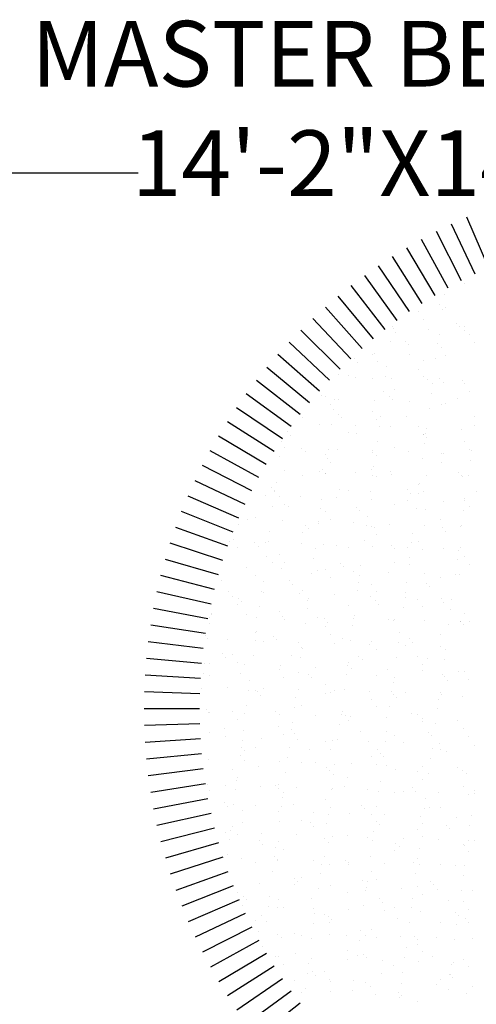
# Model space of a CAD drawing. Units: inches. Extents: x 1566 to 2546, y 1087 to 2705.
# Tile 16 of 27: x 2315 to 2364, y 1243 to 1348. Entities that reach past the tile are written whole.
import ezdxf

# ---------------------------------------------------------------- set-up
doc = ezdxf.new("R2010")
doc.units = ezdxf.units.IN
for name, color, linetype, lineweight in [('A-ANNO-DIMS', 2, 'Continuous', 18), ('A-AREA-IDEN', 7, 'Continuous', 18), ('A-FURN', 8, 'Continuous', 18)]:
    doc.layers.add(name, color=color, linetype=linetype, lineweight=lineweight)
doc.layers.add('A-HT', color=15, linetype='Continuous')
doc.styles.get("Standard").update_dxf_attribs({"font": 'arial.ttf'})
doc.dimstyles.new('ISO-25', dxfattribs={"dimtxt": 2.5, "dimasz": 2.5, "dimexe": 1.25, "dimexo": 0.625, "dimtad": 1, "dimtxsty": 'Standard', "dimcen": 2.5, "dimadec": 0, "dimazin": 0, "dimtfac": 1, "dimtmove": 0, "dimatfit": 3, "dimfxl": 1, "dimarcsym": 0})

# ---------------------------------------------------------------- blocks, each defined once
blk = doc.blocks.new('*X21')
at = {"color": 0}
for p, q in [((1.8017, 2.833), (1.8017, 2.833)), ((1.8104, 2.8275), (1.8104, 2.8275)), ((1.8783, 2.8364), (1.8783, 2.8364)), ((1.9044, 2.8399), (1.9044, 2.8399)), ((1.945, 2.8452), (1.945, 2.8452)), ((2.0018, 2.8313), (2.0018, 2.8313)), ((2.2048, 2.8269), (2.2048, 2.8269)), ((1.7428, 2.8186), (1.7428, 2.8186)), ((1.7438, 2.8187), (1.7438, 2.8187)), ((1.7537, 2.8227), (1.7537, 2.8227)), ((1.7698, 2.8221), (1.7698, 2.8221)), ((1.8778, 2.8235), (1.8778, 2.8235)), ((1.9094, 2.823), (1.9094, 2.823)), ((2.0087, 2.8252), (2.0087, 2.8252)), ((2.011, 2.8229), (2.011, 2.8229)), ((2.0652, 2.8233), (2.0652, 2.8233)), ((2.1366, 2.8246), (2.1366, 2.8246)), ((2.2209, 2.8236), (2.2209, 2.8236)), ((1.6514, 2.7891), (1.6514, 2.7891)), ((1.8133, 2.774), (1.8133, 2.774)), ((1.8515, 2.7874), (1.8515, 2.7874)), ((1.8607, 2.779), (1.8607, 2.779)), ((1.9412, 2.7734), (1.9412, 2.7734)), ((2.0545, 2.783), (2.0545, 2.783)), ((2.0763, 2.7783), (2.0763, 2.7783)), ((2.2072, 2.78), (2.2072, 2.78)), ((2.2546, 2.7813), (2.2546, 2.7813)), ((2.2638, 2.7728), (2.2638, 2.7728)), ((2.3351, 2.7793), (2.3351, 2.7793)), ((2.3949, 2.775), (2.3949, 2.775)), ((1.5414, 2.759), (1.5414, 2.759)), ((1.5474, 2.7675), (1.5474, 2.7675)), ((1.6825, 2.7724), (1.6825, 2.7724)), ((1.6971, 2.7593), (1.6971, 2.7593)), ((1.7182, 2.7459), (1.7182, 2.7459)), ((1.8528, 2.7596), (1.8528, 2.7596)), ((1.8739, 2.7462), (1.8739, 2.7462)), ((2.0085, 2.7599), (2.0085, 2.7599)), ((2.0296, 2.7465), (2.0296, 2.7465)), ((2.1643, 2.7602), (2.1643, 2.7602)), ((2.1853, 2.7467), (2.1853, 2.7467)), ((2.1936, 2.7485), (2.1936, 2.7485)), ((2.2196, 2.7519), (2.2196, 2.7519)), ((2.2603, 2.7573), (2.2603, 2.7573)), ((2.32, 2.7605), (2.32, 2.7605)), ((2.3282, 2.7662), (2.3282, 2.7662)), ((2.341, 2.747), (2.341, 2.747)), ((2.3542, 2.7696), (2.3542, 2.7696)), ((2.4967, 2.7473), (2.4967, 2.7473)), ((1.4871, 2.7212), (1.4871, 2.7212)), ((1.5011, 2.7453), (1.5011, 2.7453)), ((1.5625, 2.7456), (1.5625, 2.7456)), ((1.618, 2.7229), (1.618, 2.7229)), ((1.7012, 2.7435), (1.7012, 2.7435)), ((1.7104, 2.7351), (1.7104, 2.7351)), ((1.7459, 2.7223), (1.7459, 2.7223)), ((1.881, 2.7272), (1.881, 2.7272)), ((1.9042, 2.7391), (1.9042, 2.7391)), ((1.9911, 2.7218), (1.9911, 2.7218)), ((2.0118, 2.7288), (2.0118, 2.7288)), ((2.059, 2.7308), (2.059, 2.7308)), ((2.0851, 2.7342), (2.0851, 2.7342)), ((2.1043, 2.7374), (2.1043, 2.7374)), ((2.1135, 2.729), (2.1135, 2.729)), ((2.1257, 2.7395), (2.1257, 2.7395)), ((2.1397, 2.7282), (2.1397, 2.7282)), ((2.2748, 2.7331), (2.2748, 2.7331)), ((2.3073, 2.733), (2.3073, 2.733)), ((2.4057, 2.7348), (2.4057, 2.7348)), ((2.5074, 2.7313), (2.5074, 2.7313)), ((2.5166, 2.7228), (2.5166, 2.7228)), ((2.5336, 2.7341), (2.5336, 2.7341)), ((1.4827, 2.697), (1.4827, 2.697)), ((1.5509, 2.6997), (1.5509, 2.6997)), ((1.6384, 2.6973), (1.6384, 2.6973)), ((1.7539, 2.6952), (1.7539, 2.6952)), ((1.7899, 2.6953), (1.7899, 2.6953)), ((1.7941, 2.6975), (1.7941, 2.6975)), ((1.8159, 2.6988), (1.8159, 2.6988)), ((1.8565, 2.7041), (1.8565, 2.7041)), ((1.9244, 2.7131), (1.9244, 2.7131)), ((1.9498, 2.6978), (1.9498, 2.6978)), ((1.9505, 2.7165), (1.9505, 2.7165)), ((1.954, 2.6935), (1.954, 2.6935)), ((2.1055, 2.6981), (2.1055, 2.6981)), ((2.2612, 2.6984), (2.2612, 2.6984)), ((2.4169, 2.6987), (2.4169, 2.6987)), ((2.5727, 2.6989), (2.5727, 2.6989)), ((1.4227, 2.6718), (1.4227, 2.6718)), ((1.5506, 2.6712), (1.5506, 2.6712)), ((1.5601, 2.6912), (1.5601, 2.6912)), ((1.5873, 2.6687), (1.5873, 2.6687)), ((1.6553, 2.6776), (1.6553, 2.6776)), ((1.6813, 2.681), (1.6813, 2.681)), ((1.6856, 2.676), (1.6856, 2.676)), ((1.7219, 2.6864), (1.7219, 2.6864)), ((1.8165, 2.6777), (1.8165, 2.6777)), ((1.9444, 2.6771), (1.9444, 2.6771)), ((1.9632, 2.6851), (1.9632, 2.6851)), ((2.0794, 2.682), (2.0794, 2.682)), ((2.157, 2.6891), (2.157, 2.6891)), ((2.2103, 2.6836), (2.2103, 2.6836)), ((2.3382, 2.683), (2.3382, 2.683)), ((2.3571, 2.6874), (2.3571, 2.6874)), ((2.3663, 2.6789), (2.3663, 2.6789)), ((2.4733, 2.6879), (2.4733, 2.6879)), ((2.5601, 2.683), (2.5601, 2.683)), ((2.5756, 2.6693), (2.5756, 2.6693)), ((2.6042, 2.6895), (2.6042, 2.6895)), ((2.6435, 2.6783), (2.6435, 2.6783)), ((1.3861, 2.6422), (1.3861, 2.6422)), ((1.4006, 2.6558), (1.4006, 2.6558)), ((1.4098, 2.6473), (1.4098, 2.6473)), ((1.4121, 2.6456), (1.4121, 2.6456)), ((1.4528, 2.651), (1.4528, 2.651)), ((1.5207, 2.6599), (1.5207, 2.6599)), ((1.5467, 2.6633), (1.5467, 2.6633)), ((1.6036, 2.6513), (1.6036, 2.6513)), ((1.8037, 2.6496), (1.8037, 2.6496)), ((1.8129, 2.6412), (1.8129, 2.6412)), ((2.0067, 2.6452), (2.0067, 2.6452)), ((2.2068, 2.6435), (2.2068, 2.6435)), ((2.3743, 2.6428), (2.3743, 2.6428)), ((2.4003, 2.6462), (2.4003, 2.6462)), ((2.441, 2.6516), (2.441, 2.6516)), ((2.5089, 2.6605), (2.5089, 2.6605)), ((2.5349, 2.664), (2.5349, 2.664)), ((2.6718, 2.6427), (2.6718, 2.6427)), ((1.2775, 2.6279), (1.2775, 2.6279)), ((1.2915, 2.6198), (1.2915, 2.6198)), ((1.3182, 2.6332), (1.3182, 2.6332)), ((1.3552, 2.62), (1.3552, 2.62)), ((1.4261, 2.6336), (1.4261, 2.6336)), ((1.4472, 2.6201), (1.4472, 2.6201)), ((1.4903, 2.6249), (1.4903, 2.6249)), ((1.5818, 2.6338), (1.5818, 2.6338)), ((1.6029, 2.6204), (1.6029, 2.6204)), ((1.6212, 2.6266), (1.6212, 2.6266)), ((1.7375, 2.6341), (1.7375, 2.6341)), ((1.7491, 2.626), (1.7491, 2.626)), ((1.7586, 2.6207), (1.7586, 2.6207)), ((1.8841, 2.6308), (1.8841, 2.6308)), ((1.8932, 2.6344), (1.8932, 2.6344)), ((1.9143, 2.621), (1.9143, 2.621)), ((2.015, 2.6325), (2.015, 2.6325)), ((2.0489, 2.6347), (2.0489, 2.6347)), ((2.07, 2.6213), (2.07, 2.6213)), ((2.1429, 2.6319), (2.1429, 2.6319)), ((2.1718, 2.6162), (2.1718, 2.6162)), ((2.2046, 2.635), (2.2046, 2.635)), ((2.216, 2.635), (2.216, 2.635)), ((2.2257, 2.6215), (2.2257, 2.6215)), ((2.2397, 2.6251), (2.2397, 2.6251)), ((2.2657, 2.6285), (2.2657, 2.6285)), ((2.2779, 2.6367), (2.2779, 2.6367)), ((2.3064, 2.6339), (2.3064, 2.6339)), ((2.3603, 2.6352), (2.3603, 2.6352)), ((2.3814, 2.6218), (2.3814, 2.6218)), ((2.4088, 2.6384), (2.4088, 2.6384)), ((2.4098, 2.6391), (2.4098, 2.6391)), ((2.516, 2.6355), (2.516, 2.6355)), ((2.5367, 2.6378), (2.5367, 2.6378)), ((2.5371, 2.6221), (2.5371, 2.6221)), ((2.6099, 2.6374), (2.6099, 2.6374)), ((2.6191, 2.6289), (2.6191, 2.6289)), ((2.6718, 2.6358), (2.6718, 2.6358)), ((2.6928, 2.6224), (2.6928, 2.6224)), ((1.2503, 2.6119), (1.2503, 2.6119)), ((1.2595, 2.6034), (1.2595, 2.6034)), ((1.4533, 2.6075), (1.4533, 2.6075)), ((1.6534, 2.6057), (1.6534, 2.6057)), ((1.6626, 2.5973), (1.6626, 2.5973)), ((1.8564, 2.6013), (1.8564, 2.6013)), ((1.9705, 2.5897), (1.9705, 2.5897)), ((1.9966, 2.5931), (1.9966, 2.5931)), ((2.0372, 2.5984), (2.0372, 2.5984)), ((2.0565, 2.5996), (2.0565, 2.5996)), ((2.0657, 2.5912), (2.0657, 2.5912)), ((2.1051, 2.6074), (2.1051, 2.6074)), ((2.1312, 2.6108), (2.1312, 2.6108)), ((2.2135, 2.5873), (2.2135, 2.5873)), ((2.2595, 2.5952), (2.2595, 2.5952)), ((2.3414, 2.5867), (2.3414, 2.5867)), ((2.4595, 2.5935), (2.4595, 2.5935)), ((2.4764, 2.5915), (2.4764, 2.5915)), ((2.6073, 2.5932), (2.6073, 2.5932)), ((2.6626, 2.589), (2.6626, 2.589)), ((2.7352, 2.5926), (2.7352, 2.5926)), ((1.2117, 2.5712), (1.2117, 2.5712)), ((1.2949, 2.5738), (1.2949, 2.5738)), ((1.303, 2.5636), (1.303, 2.5636)), ((1.3674, 2.5715), (1.3674, 2.5715)), ((1.4258, 2.5754), (1.4258, 2.5754)), ((1.5031, 2.5619), (1.5031, 2.5619)), ((1.5231, 2.5718), (1.5231, 2.5718)), ((1.5537, 2.5748), (1.5537, 2.5748)), ((1.6788, 2.572), (1.6788, 2.572)), ((1.6888, 2.5797), (1.6888, 2.5797)), ((1.768, 2.563), (1.768, 2.563)), ((1.8196, 2.5814), (1.8196, 2.5814)), ((1.8345, 2.5723), (1.8345, 2.5723)), ((1.836, 2.5719), (1.836, 2.5719)), ((1.862, 2.5754), (1.862, 2.5754)), ((1.9026, 2.5807), (1.9026, 2.5807)), ((1.9475, 2.5807), (1.9475, 2.5807)), ((1.9902, 2.5726), (1.9902, 2.5726)), ((2.0826, 2.5856), (2.0826, 2.5856)), ((2.1459, 2.5729), (2.1459, 2.5729)), ((2.3016, 2.5732), (2.3016, 2.5732)), ((2.4573, 2.5735), (2.4573, 2.5735)), ((2.4688, 2.585), (2.4688, 2.585)), ((2.613, 2.5737), (2.613, 2.5737)), ((2.7563, 2.5636), (2.7563, 2.5636)), ((2.7687, 2.574), (2.7687, 2.574)), ((1.5123, 2.5534), (1.5123, 2.5534)), ((1.5668, 2.5365), (1.5668, 2.5365)), ((1.5928, 2.5399), (1.5928, 2.5399)), ((1.6334, 2.5453), (1.6334, 2.5453)), ((1.7014, 2.5542), (1.7014, 2.5542)), ((1.7061, 2.5574), (1.7061, 2.5574)), ((1.7274, 2.5577), (1.7274, 2.5577)), ((1.8873, 2.5345), (1.8873, 2.5345)), ((1.9061, 2.5557), (1.9061, 2.5557)), ((1.9154, 2.5473), (1.9154, 2.5473)), ((2.0181, 2.5361), (2.0181, 2.5361)), ((2.1092, 2.5513), (2.1092, 2.5513)), ((2.146, 2.5355), (2.146, 2.5355)), ((2.2811, 2.5404), (2.2811, 2.5404)), ((2.3092, 2.5496), (2.3092, 2.5496)), ((2.3185, 2.5411), (2.3185, 2.5411)), ((2.412, 2.5421), (2.412, 2.5421)), ((2.5123, 2.5452), (2.5123, 2.5452)), ((2.5399, 2.5415), (2.5399, 2.5415)), ((2.555, 2.5371), (2.555, 2.5371)), ((2.581, 2.5406), (2.581, 2.5406)), ((2.6217, 2.5459), (2.6217, 2.5459)), ((2.6749, 2.5463), (2.6749, 2.5463)), ((2.6896, 2.5549), (2.6896, 2.5549)), ((2.7123, 2.5434), (2.7123, 2.5434)), ((2.7156, 2.5583), (2.7156, 2.5583)), ((2.7216, 2.535), (2.7216, 2.535)), ((1.1527, 2.5197), (1.1527, 2.5197)), ((1.1551, 2.5078), (1.1551, 2.5078)), ((1.2305, 2.5243), (1.2305, 2.5243)), ((1.3108, 2.5081), (1.3108, 2.5081)), ((1.3527, 2.518), (1.3527, 2.518)), ((1.3584, 2.5237), (1.3584, 2.5237)), ((1.362, 2.5095), (1.362, 2.5095)), ((1.3643, 2.5098), (1.3643, 2.5098)), ((1.4322, 2.5188), (1.4322, 2.5188)), ((1.4582, 2.5222), (1.4582, 2.5222)), ((1.4665, 2.5083), (1.4665, 2.5083)), ((1.4934, 2.5286), (1.4934, 2.5286)), ((1.4989, 2.5276), (1.4989, 2.5276)), ((1.5558, 2.5136), (1.5558, 2.5136)), ((1.6222, 2.5086), (1.6222, 2.5086)), ((1.6243, 2.5302), (1.6243, 2.5302)), ((1.7522, 2.5296), (1.7522, 2.5296)), ((1.7558, 2.5118), (1.7558, 2.5118)), ((1.7779, 2.5089), (1.7779, 2.5089)), ((1.9336, 2.5092), (1.9336, 2.5092)), ((1.9589, 2.5074), (1.9589, 2.5074)), ((2.0893, 2.5095), (2.0893, 2.5095)), ((2.245, 2.5098), (2.245, 2.5098)), ((2.3525, 2.5105), (2.3525, 2.5105)), ((2.4007, 2.51), (2.4007, 2.51)), ((2.4204, 2.5194), (2.4204, 2.5194)), ((2.4464, 2.5229), (2.4464, 2.5229)), ((2.4871, 2.5282), (2.4871, 2.5282)), ((2.5564, 2.5103), (2.5564, 2.5103)), ((2.7121, 2.5106), (2.7121, 2.5106)), ((1.163, 2.4833), (1.163, 2.4833)), ((1.1761, 2.4943), (1.1761, 2.4943)), ((1.189, 2.4868), (1.189, 2.4868)), ((1.2297, 2.4921), (1.2297, 2.4921)), ((1.2976, 2.5011), (1.2976, 2.5011)), ((1.3236, 2.5045), (1.3236, 2.5045)), ((1.3319, 2.4946), (1.3319, 2.4946)), ((1.4876, 2.4949), (1.4876, 2.4949)), ((1.6433, 2.4952), (1.6433, 2.4952)), ((1.6919, 2.4833), (1.6919, 2.4833)), ((1.7651, 2.5034), (1.7651, 2.5034)), ((1.799, 2.4955), (1.799, 2.4955)), ((1.8228, 2.485), (1.8228, 2.485)), ((1.9507, 2.4844), (1.9507, 2.4844)), ((1.9547, 2.4958), (1.9547, 2.4958)), ((2.0857, 2.4893), (2.0857, 2.4893)), ((2.1104, 2.496), (2.1104, 2.496)), ((2.1512, 2.484), (2.1512, 2.484)), ((2.1589, 2.5057), (2.1589, 2.5057)), ((2.1682, 2.4973), (2.1682, 2.4973)), ((2.1773, 2.4874), (2.1773, 2.4874)), ((2.2166, 2.4909), (2.2166, 2.4909)), ((2.2179, 2.4928), (2.2179, 2.4928)), ((2.2661, 2.4963), (2.2661, 2.4963)), ((2.2858, 2.5017), (2.2858, 2.5017)), ((2.3118, 2.5051), (2.3118, 2.5051)), ((2.3445, 2.4903), (2.3445, 2.4903)), ((2.362, 2.5013), (2.362, 2.5013)), ((2.4218, 2.4966), (2.4218, 2.4966)), ((2.4796, 2.4952), (2.4796, 2.4952)), ((2.562, 2.4996), (2.562, 2.4996)), ((2.5712, 2.4911), (2.5712, 2.4911)), ((2.5775, 2.4969), (2.5775, 2.4969)), ((2.6104, 2.4969), (2.6104, 2.4969)), ((2.7332, 2.4972), (2.7332, 2.4972)), ((2.7384, 2.4962), (2.7384, 2.4962)), ((2.7651, 2.4951), (2.7651, 2.4951)), ((1.0951, 2.4744), (1.0951, 2.4744)), ((1.163, 2.4726), (1.163, 2.4726)), ((1.2024, 2.4741), (1.2024, 2.4741)), ((1.2117, 2.4657), (1.2117, 2.4657)), ((1.2981, 2.4774), (1.2981, 2.4774)), ((1.4055, 2.4697), (1.4055, 2.4697)), ((1.429, 2.4791), (1.429, 2.4791)), ((1.5569, 2.4785), (1.5569, 2.4785)), ((1.6055, 2.468), (1.6055, 2.468)), ((1.6148, 2.4595), (1.6148, 2.4595)), ((1.8086, 2.4635), (1.8086, 2.4635)), ((1.9487, 2.4573), (1.9487, 2.4573)), ((2.0086, 2.4618), (2.0086, 2.4618)), ((2.0166, 2.4663), (2.0166, 2.4663)), ((2.0178, 2.4534), (2.0178, 2.4534)), ((2.0427, 2.4697), (2.0427, 2.4697)), ((2.0833, 2.4751), (2.0833, 2.4751)), ((2.2117, 2.4574), (2.2117, 2.4574)), ((2.4117, 2.4557), (2.4117, 2.4557)), ((1.0521, 2.4302), (1.0521, 2.4302)), ((1.0963, 2.4457), (1.0963, 2.4457)), ((1.1027, 2.4263), (1.1027, 2.4263)), ((1.2336, 2.428), (1.2336, 2.428)), ((1.2521, 2.446), (1.2521, 2.446)), ((1.3615, 2.4273), (1.3615, 2.4273)), ((1.4078, 2.4463), (1.4078, 2.4463)), ((1.4966, 2.4322), (1.4966, 2.4322)), ((1.5635, 2.4466), (1.5635, 2.4466)), ((1.6275, 2.4339), (1.6275, 2.4339)), ((1.7192, 2.4468), (1.7192, 2.4468)), ((1.7475, 2.4308), (1.7475, 2.4308)), ((1.7554, 2.4333), (1.7554, 2.4333)), ((1.7735, 2.4343), (1.7735, 2.4343)), ((1.8141, 2.4396), (1.8141, 2.4396)), ((1.8749, 2.4471), (1.8749, 2.4471)), ((1.8821, 2.4486), (1.8821, 2.4486)), ((1.8904, 2.4381), (1.8904, 2.4381)), ((1.9081, 2.452), (1.9081, 2.452)), ((2.0213, 2.4398), (2.0213, 2.4398)), ((2.0306, 2.4474), (2.0306, 2.4474)), ((2.1492, 2.4392), (2.1492, 2.4392)), ((2.1863, 2.4477), (2.1863, 2.4477)), ((2.2842, 2.4441), (2.2842, 2.4441)), ((2.342, 2.448), (2.342, 2.448)), ((2.4151, 2.4457), (2.4151, 2.4457)), ((2.4209, 2.4472), (2.4209, 2.4472)), ((2.4977, 2.4483), (2.4977, 2.4483)), ((2.543, 2.4451), (2.543, 2.4451)), ((2.6147, 2.4513), (2.6147, 2.4513)), ((2.6534, 2.4485), (2.6534, 2.4485)), ((2.6781, 2.45), (2.6781, 2.45)), ((2.7357, 2.4315), (2.7357, 2.4315)), ((2.7617, 2.4349), (2.7617, 2.4349)), ((1.0613, 2.4218), (1.0613, 2.4218)), ((1.2552, 2.4258), (1.2552, 2.4258)), ((1.4552, 2.4241), (1.4552, 2.4241)), ((1.4644, 2.4156), (1.4644, 2.4156)), ((1.545, 2.4042), (1.545, 2.4042)), ((1.6129, 2.4131), (1.6129, 2.4131)), ((1.6389, 2.4165), (1.6389, 2.4165)), ((1.6582, 2.4197), (1.6582, 2.4197)), ((1.6795, 2.4219), (1.6795, 2.4219)), ((1.8583, 2.4179), (1.8583, 2.4179)), ((1.8675, 2.4095), (1.8675, 2.4095)), ((2.0613, 2.4135), (2.0613, 2.4135)), ((2.2614, 2.4118), (2.2614, 2.4118)), ((2.2706, 2.4033), (2.2706, 2.4033)), ((2.4644, 2.4074), (2.4644, 2.4074)), ((2.4925, 2.3995), (2.4925, 2.3995)), ((2.5332, 2.4048), (2.5332, 2.4048)), ((2.6011, 2.4138), (2.6011, 2.4138)), ((2.6136, 2.4005), (2.6136, 2.4005)), ((2.6271, 2.4172), (2.6271, 2.4172)), ((2.6645, 2.4057), (2.6645, 2.4057)), ((2.6678, 2.4225), (2.6678, 2.4225)), ((2.7415, 2.3999), (2.7415, 2.3999)), ((1.0383, 2.3768), (1.0383, 2.3768)), ((1.0397, 2.3823), (1.0397, 2.3823)), ((1.1048, 2.3819), (1.1048, 2.3819)), ((1.1662, 2.3762), (1.1662, 2.3762)), ((1.1954, 2.3826), (1.1954, 2.3826)), ((1.3012, 2.3811), (1.3012, 2.3811)), ((1.3049, 2.3802), (1.3049, 2.3802)), ((1.3437, 2.3777), (1.3437, 2.3777)), ((1.3512, 2.3829), (1.3512, 2.3829)), ((1.3697, 2.3811), (1.3697, 2.3811)), ((1.4104, 2.3865), (1.4104, 2.3865)), ((1.4321, 2.3828), (1.4321, 2.3828)), ((1.4783, 2.3954), (1.4783, 2.3954)), ((1.5043, 2.3988), (1.5043, 2.3988)), ((1.5069, 2.3831), (1.5069, 2.3831)), ((1.5079, 2.3758), (1.5079, 2.3758)), ((1.56, 2.3821), (1.56, 2.3821)), ((1.6626, 2.3834), (1.6626, 2.3834)), ((1.6951, 2.387), (1.6951, 2.387)), ((1.708, 2.374), (1.708, 2.374)), ((1.8183, 2.3837), (1.8183, 2.3837)), ((1.8259, 2.3887), (1.8259, 2.3887)), ((1.9538, 2.3881), (1.9538, 2.3881)), ((1.974, 2.384), (1.974, 2.384)), ((2.0889, 2.3929), (2.0889, 2.3929)), ((2.1297, 2.3843), (2.1297, 2.3843)), ((2.2198, 2.3946), (2.2198, 2.3946)), ((2.2854, 2.3846), (2.2854, 2.3846)), ((2.3319, 2.3783), (2.3319, 2.3783)), ((2.3477, 2.394), (2.3477, 2.394)), ((2.3579, 2.3817), (2.3579, 2.3817)), ((2.3986, 2.3871), (2.3986, 2.3871)), ((2.4411, 2.3848), (2.4411, 2.3848)), ((2.4665, 2.396), (2.4665, 2.396)), ((2.4827, 2.3988), (2.4827, 2.3988)), ((2.5968, 2.3851), (2.5968, 2.3851)), ((2.6737, 2.3972), (2.6737, 2.3972)), ((2.7525, 2.3854), (2.7525, 2.3854)), ((1.0608, 2.3689), (1.0608, 2.3689)), ((1.1412, 2.351), (1.1412, 2.351)), ((1.2091, 2.36), (1.2091, 2.36)), ((1.2165, 2.3691), (1.2165, 2.3691)), ((1.2351, 2.3634), (1.2351, 2.3634)), ((1.2758, 2.3687), (1.2758, 2.3687)), ((1.3141, 2.3717), (1.3141, 2.3717)), ((1.3722, 2.3694), (1.3722, 2.3694)), ((1.5279, 2.3697), (1.5279, 2.3697)), ((1.6837, 2.37), (1.6837, 2.37)), ((1.7172, 2.3656), (1.7172, 2.3656)), ((1.8394, 2.3703), (1.8394, 2.3703)), ((1.911, 2.3696), (1.911, 2.3696)), ((1.9951, 2.3706), (1.9951, 2.3706)), ((2.0888, 2.3463), (2.0888, 2.3463)), ((2.1111, 2.3679), (2.1111, 2.3679)), ((2.1203, 2.3595), (2.1203, 2.3595)), ((2.1294, 2.3517), (2.1294, 2.3517)), ((2.1508, 2.3708), (2.1508, 2.3708)), ((2.1973, 2.3606), (2.1973, 2.3606)), ((2.2234, 2.364), (2.2234, 2.364)), ((2.264, 2.3694), (2.264, 2.3694)), ((2.2874, 2.3477), (2.2874, 2.3477)), ((2.3065, 2.3711), (2.3065, 2.3711)), ((2.3141, 2.3635), (2.3141, 2.3635)), ((2.4183, 2.3494), (2.4183, 2.3494)), ((2.4622, 2.3714), (2.4622, 2.3714)), ((2.5142, 2.3618), (2.5142, 2.3618)), ((2.5234, 2.3533), (2.5234, 2.3533)), ((2.5462, 2.3488), (2.5462, 2.3488)), ((2.6179, 2.3717), (2.6179, 2.3717)), ((2.6812, 2.3536), (2.6812, 2.3536)), ((2.7172, 2.3573), (2.7172, 2.3573)), ((2.7736, 2.372), (2.7736, 2.372)), ((0.966, 2.3279), (0.966, 2.3279)), ((0.9708, 2.3251), (0.9708, 2.3251)), ((0.981, 2.3202), (0.981, 2.3202)), ((1.0066, 2.3333), (1.0066, 2.3333)), ((1.0745, 2.3422), (1.0745, 2.3422)), ((1.1005, 2.3457), (1.1005, 2.3457)), ((1.1059, 2.33), (1.1059, 2.33)), ((1.1367, 2.3205), (1.1367, 2.3205)), ((1.1546, 2.3363), (1.1546, 2.3363)), ((1.1638, 2.3279), (1.1638, 2.3279)), ((1.2368, 2.3316), (1.2368, 2.3316)), ((1.2924, 2.3208), (1.2924, 2.3208)), ((1.3576, 2.3319), (1.3576, 2.3319)), ((1.3647, 2.331), (1.3647, 2.331)), ((1.4481, 2.3211), (1.4481, 2.3211)), ((1.4997, 2.3359), (1.4997, 2.3359)), ((1.5577, 2.3302), (1.5577, 2.3302)), ((1.5669, 2.3217), (1.5669, 2.3217)), ((1.6038, 2.3214), (1.6038, 2.3214)), ((1.6306, 2.3375), (1.6306, 2.3375)), ((1.7585, 2.3369), (1.7585, 2.3369)), ((1.7596, 2.3216), (1.7596, 2.3216)), ((1.7607, 2.3257), (1.7607, 2.3257)), ((1.8936, 2.3418), (1.8936, 2.3418)), ((1.9153, 2.3219), (1.9153, 2.3219)), ((1.9282, 2.3252), (1.9282, 2.3252)), ((1.9542, 2.3286), (1.9542, 2.3286)), ((1.9608, 2.324), (1.9608, 2.324)), ((1.9948, 2.3339), (1.9948, 2.3339)), ((2.0244, 2.3435), (2.0244, 2.3435)), ((2.0627, 2.3429), (2.0627, 2.3429)), ((2.071, 2.3222), (2.071, 2.3222)), ((2.1523, 2.3429), (2.1523, 2.3429)), ((2.1638, 2.3196), (2.1638, 2.3196)), ((2.2267, 2.3225), (2.2267, 2.3225)), ((2.3824, 2.3228), (2.3824, 2.3228)), ((2.5381, 2.323), (2.5381, 2.323)), ((2.6938, 2.3233), (2.6938, 2.3233)), ((1.685, 2.2932), (1.685, 2.2932)), ((1.7256, 2.2985), (1.7256, 2.2985)), ((1.7936, 2.3074), (1.7936, 2.3074)), ((1.8196, 2.3109), (1.8196, 2.3109)), ((1.8602, 2.3162), (1.8602, 2.3162)), ((1.97, 2.3156), (1.97, 2.3156)), ((2.092, 2.2966), (2.092, 2.2966)), ((2.2229, 2.2983), (2.2229, 2.2983)), ((2.3508, 2.2976), (2.3508, 2.2976)), ((2.3639, 2.3179), (2.3639, 2.3179)), ((2.3731, 2.3094), (2.3731, 2.3094)), ((2.4859, 2.3025), (2.4859, 2.3025)), ((2.5669, 2.3135), (2.5669, 2.3135)), ((2.6167, 2.3042), (2.6167, 2.3042)), ((2.6732, 2.2938), (2.6732, 2.2938)), ((2.7139, 2.2992), (2.7139, 2.2992)), ((2.7447, 2.3036), (2.7447, 2.3036)), ((2.767, 2.3117), (2.767, 2.3117)), ((2.7762, 2.3033), (2.7762, 2.3033)), ((2.7818, 2.3081), (2.7818, 2.3081)), ((1.0043, 2.2924), (1.0043, 2.2924)), ((1.0135, 2.284), (1.0135, 2.284)), ((1.0414, 2.2805), (1.0414, 2.2805)), ((1.1693, 2.2799), (1.1693, 2.2799)), ((1.2073, 2.288), (1.2073, 2.288)), ((1.3044, 2.2847), (1.3044, 2.2847)), ((1.4074, 2.2863), (1.4074, 2.2863)), ((1.4166, 2.2778), (1.4166, 2.2778)), ((1.4353, 2.2864), (1.4353, 2.2864)), ((1.5244, 2.272), (1.5244, 2.272)), ((1.5504, 2.2754), (1.5504, 2.2754)), ((1.5632, 2.2858), (1.5632, 2.2858)), ((1.5911, 2.2808), (1.5911, 2.2808)), ((1.6104, 2.2819), (1.6104, 2.2819)), ((1.659, 2.2897), (1.659, 2.2897)), ((1.6982, 2.2907), (1.6982, 2.2907)), ((1.8105, 2.2801), (1.8105, 2.2801)), ((1.8197, 2.2717), (1.8197, 2.2717)), ((1.8291, 2.2923), (1.8291, 2.2923)), ((1.957, 2.2917), (1.957, 2.2917)), ((2.0135, 2.2757), (2.0135, 2.2757)), ((2.2136, 2.274), (2.2136, 2.274)), ((2.4166, 2.2696), (2.4166, 2.2696)), ((2.5126, 2.2727), (2.5126, 2.2727)), ((2.5386, 2.2761), (2.5386, 2.2761)), ((2.5793, 2.2814), (2.5793, 2.2814)), ((2.6167, 2.2679), (2.6167, 2.2679)), ((2.6472, 2.2904), (2.6472, 2.2904)), ((0.9244, 2.2568), (0.9244, 2.2568)), ((0.9455, 2.2434), (0.9455, 2.2434)), ((1.057, 2.2441), (1.057, 2.2441)), ((1.0801, 2.2571), (1.0801, 2.2571)), ((1.1012, 2.2437), (1.1012, 2.2437)), ((1.2358, 2.2574), (1.2358, 2.2574)), ((1.2569, 2.2439), (1.2569, 2.2439)), ((1.2571, 2.2424), (1.2571, 2.2424)), ((1.2812, 2.24), (1.2812, 2.24)), ((1.3219, 2.2453), (1.3219, 2.2453)), ((1.3898, 2.2543), (1.3898, 2.2543)), ((1.3915, 2.2577), (1.3915, 2.2577)), ((1.4126, 2.2442), (1.4126, 2.2442)), ((1.4158, 2.2577), (1.4158, 2.2577)), ((1.4565, 2.2631), (1.4565, 2.2631)), ((1.5029, 2.2395), (1.5029, 2.2395)), ((1.5472, 2.2579), (1.5472, 2.2579)), ((1.5683, 2.2445), (1.5683, 2.2445)), ((1.6338, 2.2412), (1.6338, 2.2412)), ((1.7029, 2.2582), (1.7029, 2.2582)), ((1.724, 2.2448), (1.724, 2.2448)), ((1.7617, 2.2406), (1.7617, 2.2406)), ((1.8587, 2.2585), (1.8587, 2.2585)), ((1.8797, 2.2451), (1.8797, 2.2451)), ((1.8967, 2.2455), (1.8967, 2.2455)), ((2.0144, 2.2588), (2.0144, 2.2588)), ((2.0276, 2.2471), (2.0276, 2.2471)), ((2.0354, 2.2454), (2.0354, 2.2454)), ((2.1555, 2.2465), (2.1555, 2.2465)), ((2.1701, 2.2591), (2.1701, 2.2591)), ((2.1912, 2.2456), (2.1912, 2.2456)), ((2.2228, 2.2656), (2.2228, 2.2656)), ((2.2695, 2.2406), (2.2695, 2.2406)), ((2.2905, 2.2514), (2.2905, 2.2514)), ((2.3101, 2.246), (2.3101, 2.246)), ((2.3258, 2.2594), (2.3258, 2.2594)), ((2.3469, 2.2459), (2.3469, 2.2459)), ((2.378, 2.2549), (2.378, 2.2549)), ((2.404, 2.2584), (2.404, 2.2584)), ((2.4214, 2.253), (2.4214, 2.253)), ((2.4447, 2.2637), (2.4447, 2.2637)), ((2.4815, 2.2596), (2.4815, 2.2596)), ((2.5026, 2.2462), (2.5026, 2.2462)), ((2.5493, 2.2524), (2.5493, 2.2524)), ((2.6259, 2.2594), (2.6259, 2.2594)), ((2.6372, 2.2599), (2.6372, 2.2599)), ((2.6583, 2.2465), (2.6583, 2.2465)), ((2.6844, 2.2573), (2.6844, 2.2573)), ((2.7929, 2.2602), (2.7929, 2.2602)), ((0.974, 2.2287), (0.974, 2.2287)), ((1.109, 2.2336), (1.109, 2.2336)), ((1.1206, 2.2189), (1.1206, 2.2189)), ((1.1466, 2.2223), (1.1466, 2.2223)), ((1.1873, 2.2276), (1.1873, 2.2276)), ((1.2399, 2.2353), (1.2399, 2.2353)), ((1.2552, 2.2366), (1.2552, 2.2366)), ((1.2663, 2.234), (1.2663, 2.234)), ((1.3678, 2.2347), (1.3678, 2.2347)), ((1.4601, 2.238), (1.4601, 2.238)), ((1.6602, 2.2363), (1.6602, 2.2363)), ((1.6694, 2.2278), (1.6694, 2.2278)), ((1.8632, 2.2318), (1.8632, 2.2318)), ((2.0633, 2.2301), (2.0633, 2.2301)), ((2.0725, 2.2217), (2.0725, 2.2217)), ((2.1088, 2.2195), (2.1088, 2.2195)), ((2.1349, 2.2229), (2.1349, 2.2229)), ((2.1755, 2.2283), (2.1755, 2.2283)), ((2.2434, 2.2372), (2.2434, 2.2372)), ((2.2663, 2.2257), (2.2663, 2.2257)), ((2.4664, 2.224), (2.4664, 2.224)), ((2.4756, 2.2155), (2.4756, 2.2155)), ((2.6694, 2.2196), (2.6694, 2.2196)), ((0.8775, 2.1868), (0.8775, 2.1868)), ((0.9067, 2.2002), (0.9067, 2.2002)), ((0.9181, 2.1922), (0.9181, 2.1922)), ((0.986, 2.2011), (0.986, 2.2011)), ((1.0121, 2.2046), (1.0121, 2.2046)), ((1.0214, 2.195), (1.0214, 2.195)), ((1.0527, 2.2099), (1.0527, 2.2099)), ((1.1068, 2.1985), (1.1068, 2.1985)), ((1.116, 2.1901), (1.116, 2.1901)), ((1.1771, 2.1953), (1.1771, 2.1953)), ((1.3075, 2.1884), (1.3075, 2.1884)), ((1.3098, 2.1941), (1.3098, 2.1941)), ((1.3328, 2.1956), (1.3328, 2.1956)), ((1.4384, 2.1901), (1.4384, 2.1901)), ((1.4885, 2.1959), (1.4885, 2.1959)), ((1.5099, 2.1924), (1.5099, 2.1924)), ((1.5663, 2.1895), (1.5663, 2.1895)), ((1.6442, 2.1961), (1.6442, 2.1961)), ((1.7014, 2.1943), (1.7014, 2.1943)), ((1.7129, 2.188), (1.7129, 2.188)), ((1.7999, 2.1964), (1.7999, 2.1964)), ((1.8322, 2.196), (1.8322, 2.196)), ((1.8657, 2.1875), (1.8657, 2.1875)), ((1.9063, 2.1928), (1.9063, 2.1928)), ((1.913, 2.1862), (1.913, 2.1862)), ((1.9556, 2.1967), (1.9556, 2.1967)), ((1.9601, 2.1954), (1.9601, 2.1954)), ((1.9743, 2.2018), (1.9743, 2.2018)), ((2.0003, 2.2052), (2.0003, 2.2052)), ((2.0409, 2.2106), (2.0409, 2.2106)), ((2.0952, 2.2002), (2.0952, 2.2002)), ((2.1114, 2.197), (2.1114, 2.197)), ((2.2261, 2.2019), (2.2261, 2.2019)), ((2.2671, 2.1973), (2.2671, 2.1973)), ((2.354, 2.2013), (2.354, 2.2013)), ((2.4228, 2.1976), (2.4228, 2.1976)), ((2.489, 2.2062), (2.489, 2.2062)), ((2.5785, 2.1978), (2.5785, 2.1978)), ((2.6199, 2.2078), (2.6199, 2.2078)), ((2.7342, 2.1981), (2.7342, 2.1981)), ((2.7478, 2.2072), (2.7478, 2.2072)), ((0.9137, 2.1825), (0.9137, 2.1825)), ((1.0446, 2.1841), (1.0446, 2.1841)), ((1.1725, 2.1835), (1.1725, 2.1835)), ((1.5191, 2.1839), (1.5191, 2.1839)), ((1.7051, 2.1663), (1.7051, 2.1663)), ((1.7311, 2.1698), (1.7311, 2.1698)), ((1.7717, 2.1751), (1.7717, 2.1751)), ((1.8397, 2.1841), (1.8397, 2.1841)), ((1.9222, 2.1778), (1.9222, 2.1778)), ((2.116, 2.1818), (2.116, 2.1818)), ((2.3161, 2.1801), (2.3161, 2.1801)), ((2.3253, 2.1717), (2.3253, 2.1717)), ((2.5191, 2.1757), (2.5191, 2.1757)), ((2.6875, 2.161), (2.6875, 2.161)), ((2.6933, 2.167), (2.6933, 2.167)), ((2.7192, 2.174), (2.7192, 2.174)), ((2.7193, 2.1704), (2.7193, 2.1704)), ((2.7284, 2.1655), (2.7284, 2.1655)), ((2.76, 2.1758), (2.76, 2.1758)), ((0.8492, 2.133), (0.8492, 2.133)), ((0.9565, 2.1546), (0.9565, 2.1546)), ((0.9657, 2.1462), (0.9657, 2.1462)), ((1.1122, 2.1373), (1.1122, 2.1373)), ((1.1595, 2.1502), (1.1595, 2.1502)), ((1.2431, 2.1389), (1.2431, 2.1389)), ((1.3596, 2.1485), (1.3596, 2.1485)), ((1.3688, 2.14), (1.3688, 2.14)), ((1.371, 2.1383), (1.371, 2.1383)), ((1.4619, 2.1343), (1.4619, 2.1343)), ((1.5026, 2.1397), (1.5026, 2.1397)), ((1.506, 2.1432), (1.506, 2.1432)), ((1.5626, 2.1441), (1.5626, 2.1441)), ((1.5705, 2.1486), (1.5705, 2.1486)), ((1.5876, 2.1327), (1.5876, 2.1327)), ((1.5965, 2.152), (1.5965, 2.152)), ((1.6369, 2.1449), (1.6369, 2.1449)), ((1.6372, 2.1574), (1.6372, 2.1574)), ((1.7433, 2.133), (1.7433, 2.133)), ((1.7627, 2.1424), (1.7627, 2.1424)), ((1.7648, 2.1442), (1.7648, 2.1442)), ((1.7719, 2.1339), (1.7719, 2.1339)), ((1.899, 2.1333), (1.899, 2.1333)), ((1.8999, 2.1491), (1.8999, 2.1491)), ((1.9657, 2.1379), (1.9657, 2.1379)), ((2.0307, 2.1508), (2.0307, 2.1508)), ((2.0547, 2.1336), (2.0547, 2.1336)), ((2.1586, 2.1502), (2.1586, 2.1502)), ((2.1658, 2.1362), (2.1658, 2.1362)), ((2.2105, 2.1339), (2.2105, 2.1339)), ((2.2937, 2.155), (2.2937, 2.155)), ((2.3662, 2.1341), (2.3662, 2.1341)), ((2.4246, 2.1567), (2.4246, 2.1567)), ((2.4501, 2.135), (2.4501, 2.135)), ((2.4908, 2.1403), (2.4908, 2.1403)), ((2.5219, 2.1344), (2.5219, 2.1344)), ((2.5525, 2.1561), (2.5525, 2.1561)), ((2.5587, 2.1493), (2.5587, 2.1493)), ((2.5847, 2.1527), (2.5847, 2.1527)), ((2.6254, 2.158), (2.6254, 2.158)), ((2.6776, 2.1347), (2.6776, 2.1347)), ((0.9648, 2.1316), (0.9648, 2.1316)), ((0.9771, 2.1324), (0.9771, 2.1324)), ((0.9859, 2.1182), (0.9859, 2.1182)), ((1.0092, 2.1063), (1.0092, 2.1063)), ((1.1205, 2.1319), (1.1205, 2.1319)), ((1.1416, 2.1184), (1.1416, 2.1184)), ((1.2762, 2.1322), (1.2762, 2.1322)), ((1.2973, 2.1187), (1.2973, 2.1187)), ((1.3013, 2.1132), (1.3013, 2.1132)), ((1.3273, 2.1166), (1.3273, 2.1166)), ((1.368, 2.122), (1.368, 2.122)), ((1.4319, 2.1324), (1.4319, 2.1324)), ((1.4359, 2.1309), (1.4359, 2.1309)), ((1.453, 2.119), (1.453, 2.119)), ((1.6087, 2.1193), (1.6087, 2.1193)), ((1.7644, 2.1196), (1.7644, 2.1196)), ((1.9201, 2.1199), (1.9201, 2.1199)), ((2.0758, 2.1201), (2.0758, 2.1201)), ((2.175, 2.1278), (2.175, 2.1278)), ((2.2315, 2.1204), (2.2315, 2.1204)), ((2.2895, 2.1138), (2.2895, 2.1138)), ((2.3156, 2.1173), (2.3156, 2.1173)), ((2.3562, 2.1226), (2.3562, 2.1226)), ((2.3688, 2.1318), (2.3688, 2.1318)), ((2.3872, 2.1207), (2.3872, 2.1207)), ((2.4241, 2.1315), (2.4241, 2.1315)), ((2.4922, 2.1098), (2.4922, 2.1098)), ((2.5429, 2.121), (2.5429, 2.121)), ((2.5689, 2.1301), (2.5689, 2.1301)), ((2.5781, 2.1216), (2.5781, 2.1216)), ((2.623, 2.1115), (2.623, 2.1115)), ((2.6987, 2.1213), (2.6987, 2.1213)), ((2.751, 2.1109), (2.751, 2.1109)), ((2.7719, 2.1257), (2.7719, 2.1257)), ((1.2093, 2.1046), (1.2093, 2.1046)), ((1.2334, 2.1042), (1.2334, 2.1042)), ((1.4123, 2.1002), (1.4123, 2.1002)), ((2.0983, 2.1039), (2.0983, 2.1039)), ((2.2216, 2.1049), (2.2216, 2.1049)), ((2.2292, 2.1056), (2.2292, 2.1056)), ((2.3571, 2.105), (2.3571, 2.105))]:
    blk.add_line(p, q, dxfattribs=at)
blk = doc.blocks.new('A$C6796526C')
at = {"layer": 'A-HT'}
for p, q in [((0.2569, 0.9337), (0.1193, 0.8741)), ((0.2737, 0.8965), (0.138, 0.8326)), ((0.2917, 0.8598), (0.158, 0.7917)), ((0.3108, 0.8237), (0.1794, 0.7515)), ((0.331, 0.7882), (0.2019, 0.7119)), ((0.3524, 0.7534), (0.2257, 0.6731)), ((0.3748, 0.7193), (0.2507, 0.635)), ((0.3983, 0.6859), (0.2769, 0.5977)), ((0.4228, 0.6532), (0.3043, 0.5613)), ((0.4483, 0.6213), (0.3328, 0.5257)), ((0.4749, 0.5903), (0.3623, 0.4911)), ((0.5023, 0.5601), (0.393, 0.4574)), ((0.5308, 0.5308), (0.4247, 0.4247)), ((0.5601, 0.5023), (0.4574, 0.393)), ((0.5903, 0.4749), (0.4911, 0.3623)), ((0.6213, 0.4483), (0.5257, 0.3328)), ((0.6532, 0.4228), (0.5613, 0.3043)), ((2.2474, 0.423), (2.3394, 0.3045)), ((0.6859, 0.3983), (0.5977, 0.2769)), ((0.7193, 0.3748), (0.635, 0.2507)), ((2.1814, 0.375), (2.2657, 0.251)), ((2.2148, 0.3985), (2.303, 0.2772)), ((0.7534, 0.3524), (0.6731, 0.2257)), ((2.1472, 0.3526), (2.2276, 0.226)), ((0.7882, 0.331), (0.7119, 0.2019)), ((2.1124, 0.3313), (2.1888, 0.2022)), ((0.8237, 0.3108), (0.7515, 0.1794)), ((2.0769, 0.311), (2.1492, 0.1796)), ((0.8598, 0.2917), (0.7917, 0.158)), ((0.8965, 0.2737), (0.8326, 0.138)), ((2.0042, 0.274), (2.068, 0.1382)), ((2.0409, 0.2919), (2.109, 0.1583)), ((0.9337, 0.2569), (0.8741, 0.1193)), ((0.9714, 0.2413), (0.9162, 0.1018)), ((1.9292, 0.2415), (1.9844, 0.1021)), ((1.967, 0.2572), (2.0265, 0.1195)), ((1.0096, 0.2269), (0.9588, 0.0857)), ((1.0483, 0.2136), (1.0019, 0.071)), ((1.8517, 0.2136), (1.8981, 0.071)), ((1.891, 0.2271), (1.9418, 0.086)), ((1.0873, 0.2016), (1.0455, 0.0576)), ((1.1267, 0.1908), (1.0894, 0.0456)), ((1.7733, 0.1908), (1.8106, 0.0456)), ((1.8127, 0.2016), (1.8545, 0.0576)), ((1.1664, 0.1813), (1.1337, 0.0349)), ((1.2064, 0.173), (1.1783, 0.0257)), ((1.2466, 0.166), (1.2232, 0.0179)), ((1.2871, 0.1603), (1.2683, 0.0114)), ((1.6129, 0.1603), (1.6317, 0.0114)), ((1.6534, 0.166), (1.6768, 0.0179)), ((1.6936, 0.173), (1.7217, 0.0257)), ((1.7336, 0.1813), (1.7663, 0.0349)), ((1.3277, 0.1558), (1.3135, 0.0064)), ((1.3684, 0.1526), (1.359, 0.0029)), ((1.4092, 0.1506), (1.4045, 0.0007)), ((1.45, 0.15), (1.45, 0)), ((1.4908, 0.1506), (1.4955, 0.0007)), ((1.5316, 0.1526), (1.541, 0.0029)), ((1.5723, 0.1558), (1.5865, 0.0064))]:
    blk.add_line(p, q, dxfattribs=at)
at = {"layer": 'A-HT', "extrusion": (0, 0, -1), "zscale": -1, "rotation": 180}
blk.add_blockref('*X21', (0.55, 3), dxfattribs=at)
blk = doc.blocks.new('*D48')
at = {"layer": 'A-ANNO-DIMS', "color": 0, "lineweight": -2, "transparency": 16777216}
for p, q in [((2327.57, 1331.61), (2309.22, 1331.61)), ((2310.47, 1329.11), (2310.47, 1219.93)), ((2327.57, 1217.43), (2309.22, 1217.43))]:
    blk.add_line(p, q, dxfattribs=at)
at = {"layer": 'A-ANNO-DIMS', "color": 0, "transparency": 16777216}
for points in [[(2310.06, 1329.11), (2310.89, 1329.11), (2310.47, 1331.61)], [(2310.06, 1219.93), (2310.89, 1219.93), (2310.47, 1217.43)]]:
    blk.add_solid(points, dxfattribs=at)
at = {"layer": 'Defpoints', "color": 0, "transparency": 16777216}
for p in [(2328.19, 1331.61), (2310.47, 1217.43), (2328.19, 1217.43)]:
    blk.add_point(p, dxfattribs=at)
at = {"layer": 'A-ANNO-DIMS', "color": 0, "transparency": 16777216, "insert": (2308.57, 1274.52), "char_height": 2.5, "attachment_point": 5, "rotation": 90}
blk.add_mtext('9\'-6" TYP.', dxfattribs=at)

msp = doc.modelspace()

# ---------------------------------------------------------------- block references
at = {"layer": 'A-FURN', "xscale": 39.3701, "yscale": 39.3701, "zscale": 39.3701, "rotation": 270}
msp.add_blockref('A$C6796526C', (2328.19, 1331.61), dxfattribs=at)

# ---------------------------------------------------------------- texts
at = {"layer": 'A-AREA-IDEN', "insert": (2316.17, 1347.85), "char_height": 7, "attachment_point": 1}
msp.add_mtext_dynamic_manual_height_columns('MASTER BEDROOM\\P     14\'-2"X14\'-4"', width=111.7553, gutter_width=12.5, heights=[0], dxfattribs=at)

# ---------------------------------------------------------------- dimensions: what is measured, and where the dimension line sits
at = {"layer": 'A-ANNO-DIMS'}
dim = msp.add_linear_dim(base=(2310.47, 1217.43), p1=(2328.19, 1331.61), p2=(2328.19, 1217.43), angle=270, text='<> TYP.', dimstyle='ISO-25', override={"dimdec": 1, "dimrnd": 0, "dimzin": 1, "dimlunit": 4, "dimfrac": 2}, dxfattribs=at)
dim.commit()
dim.dimension.update_dxf_attribs({"geometry": '*D48', "text_midpoint": (2308.57, 1274.52)})

doc.saveas('drawing.dxf')
